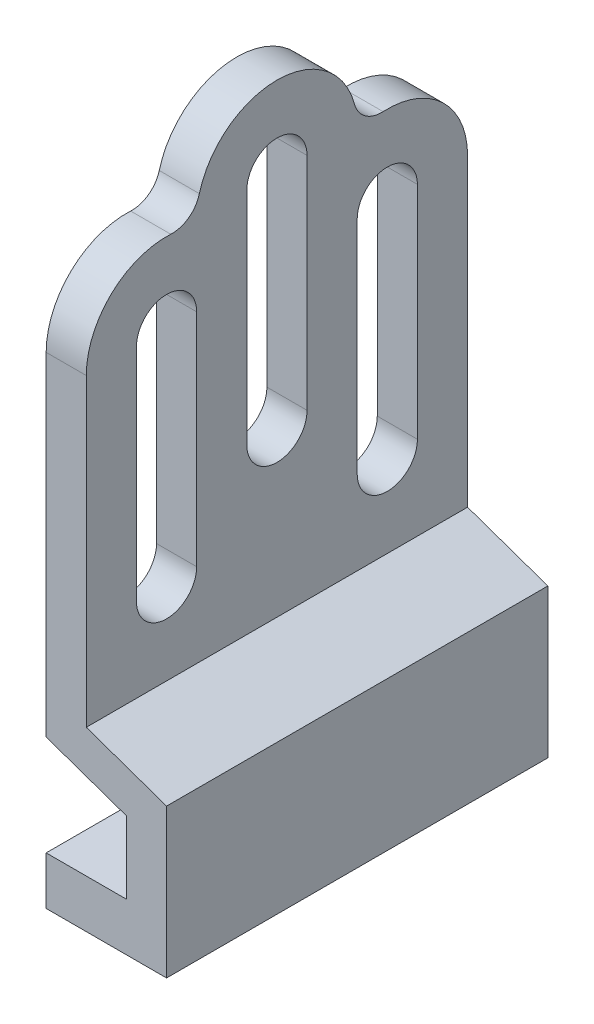
ISO-10303-21;
HEADER;
FILE_DESCRIPTION(('STEP AP214'),'2;1');
FILE_NAME('part.step','',(''),(''),'','','');
FILE_SCHEMA(('AUTOMOTIVE_DESIGN { 1 0 10303 214 1 1 1 1 }'));
ENDSEC;
DATA;
#1=APPLICATION_CONTEXT('core data for automotive mechanical design processes');
#2=APPLICATION_PROTOCOL_DEFINITION('international standard','automotive_design',2000,#1);
#3=PRODUCT_CONTEXT('',#1,'mechanical');
#4=PRODUCT('Part','Part','',(#3));
#5=PRODUCT_RELATED_PRODUCT_CATEGORY('part','',(#4));
#6=PRODUCT_DEFINITION_FORMATION('','',#4);
#7=PRODUCT_DEFINITION_CONTEXT('part definition',#1,'design');
#8=PRODUCT_DEFINITION('design','',#6,#7);
#9=PRODUCT_DEFINITION_SHAPE('','',#8);
#10=(LENGTH_UNIT() NAMED_UNIT(*) SI_UNIT(.MILLI.,.METRE.));
#11=(NAMED_UNIT(*) PLANE_ANGLE_UNIT() SI_UNIT($,.RADIAN.));
#12=(NAMED_UNIT(*) SI_UNIT($,.STERADIAN.) SOLID_ANGLE_UNIT());
#13=UNCERTAINTY_MEASURE_WITH_UNIT(LENGTH_MEASURE(1.E-05),#10,'distance_accuracy_value','');
#14=(GEOMETRIC_REPRESENTATION_CONTEXT(3) GLOBAL_UNCERTAINTY_ASSIGNED_CONTEXT((#13)) GLOBAL_UNIT_ASSIGNED_CONTEXT((#10,
#11,#12)) REPRESENTATION_CONTEXT('',''));
#15=CARTESIAN_POINT('',(0.,0.,0.));
#16=DIRECTION('',(0.,0.,1.));
#17=DIRECTION('',(1.,0.,0.));
#18=AXIS2_PLACEMENT_3D('',#15,#16,#17);
#19=CARTESIAN_POINT('',(-20.,44.0948100502085,47.5));
#20=DIRECTION('',(-1.,0.,0.));
#21=DIRECTION('',(0.,0.,1.));
#22=AXIS2_PLACEMENT_3D('',#19,#20,#21);
#23=PLANE('',#22);
#24=CARTESIAN_POINT('',(-20.,140.,0.));
#25=DIRECTION('',(1.,0.,0.));
#26=DIRECTION('',(0.,0.,-1.));
#27=AXIS2_PLACEMENT_3D('',#24,#25,#26);
#28=CIRCLE('',#27,20.);
#29=CARTESIAN_POINT('',(-20.,145.157767655643,-19.3234943219492));
#30=VERTEX_POINT('',#29);
#31=CARTESIAN_POINT('',(-20.,145.157767655643,19.3234943219492));
#32=VERTEX_POINT('',#31);
#33=EDGE_CURVE('E462',#30,#32,#28,.T.);
#34=ORIENTED_EDGE('',*,*,#33,.T.);
#35=CARTESIAN_POINT('',(-20.,146.962986335118,26.0867173346314));
#36=DIRECTION('',(1.,0.,0.));
#37=DIRECTION('',(0.,0.,-1.));
#38=AXIS2_PLACEMENT_3D('',#35,#36,#37);
#39=CIRCLE('',#38,7.);
#40=CARTESIAN_POINT('',(-20.,139.972582470458,26.4531239515788));
#41=VERTEX_POINT('',#40);
#42=EDGE_CURVE('E332',#32,#41,#39,.F.);
#43=ORIENTED_EDGE('',*,*,#42,.T.);
#44=CARTESIAN_POINT('',(-20.,120.,27.5));
#45=DIRECTION('',(1.,0.,0.));
#46=DIRECTION('',(0.,0.,-1.));
#47=AXIS2_PLACEMENT_3D('',#44,#45,#46);
#48=CIRCLE('',#47,20.);
#49=CARTESIAN_POINT('',(-20.,120.,47.5));
#50=VERTEX_POINT('',#49);
#51=EDGE_CURVE('E419',#41,#50,#48,.T.);
#52=ORIENTED_EDGE('',*,*,#51,.T.);
#53=DIRECTION('',(0.,1.,0.));
#54=VECTOR('',#53,1.);
#55=CARTESIAN_POINT('',(-20.,44.0948100502085,47.5));
#56=LINE('',#55,#54);
#57=CARTESIAN_POINT('',(-20.,44.0948100502085,47.5));
#58=VERTEX_POINT('',#57);
#59=EDGE_CURVE('E338',#58,#50,#56,.T.);
#60=ORIENTED_EDGE('',*,*,#59,.F.);
#61=DIRECTION('',(0.,0.,-1.));
#62=VECTOR('',#61,1.);
#63=CARTESIAN_POINT('',(-20.,44.0948100502085,47.5));
#64=LINE('',#63,#62);
#65=CARTESIAN_POINT('',(-20.,44.0948100502085,-47.5));
#66=VERTEX_POINT('',#65);
#67=EDGE_CURVE('E392',#58,#66,#64,.T.);
#68=ORIENTED_EDGE('',*,*,#67,.T.);
#69=DIRECTION('',(0.,1.,0.));
#70=VECTOR('',#69,1.);
#71=CARTESIAN_POINT('',(-20.,44.0948100502085,-47.5));
#72=LINE('',#71,#70);
#73=CARTESIAN_POINT('',(-20.,120.,-47.5));
#74=VERTEX_POINT('',#73);
#75=EDGE_CURVE('E367',#66,#74,#72,.T.);
#76=ORIENTED_EDGE('',*,*,#75,.T.);
#77=CARTESIAN_POINT('',(-20.,120.,-27.5));
#78=DIRECTION('',(1.,0.,0.));
#79=DIRECTION('',(0.,0.,-1.));
#80=AXIS2_PLACEMENT_3D('',#77,#78,#79);
#81=CIRCLE('',#80,20.);
#82=CARTESIAN_POINT('',(-20.,139.972582470458,-26.4531239515788));
#83=VERTEX_POINT('',#82);
#84=EDGE_CURVE('E468',#83,#74,#81,.F.);
#85=ORIENTED_EDGE('',*,*,#84,.F.);
#86=CARTESIAN_POINT('',(-20.,146.962986335118,-26.0867173346314));
#87=DIRECTION('',(1.,0.,0.));
#88=DIRECTION('',(0.,0.,-1.));
#89=AXIS2_PLACEMENT_3D('',#86,#87,#88);
#90=CIRCLE('',#89,7.);
#91=EDGE_CURVE('E464',#30,#83,#90,.T.);
#92=ORIENTED_EDGE('',*,*,#91,.F.);
#93=EDGE_LOOP('',(#34,#43,#52,#60,#68,#76,#85,#92));
#94=FACE_BOUND('',#93,.T.);
#95=CARTESIAN_POINT('',(-20.,65.,27.5));
#96=DIRECTION('',(1.,0.,0.));
#97=DIRECTION('',(0.,0.,-1.));
#98=AXIS2_PLACEMENT_3D('',#95,#96,#97);
#99=CIRCLE('',#98,7.50000000000001);
#100=CARTESIAN_POINT('',(-20.,65.,35.));
#101=VERTEX_POINT('',#100);
#102=CARTESIAN_POINT('',(-20.,65.,20.));
#103=VERTEX_POINT('',#102);
#104=EDGE_CURVE('E438',#101,#103,#99,.T.);
#105=ORIENTED_EDGE('',*,*,#104,.F.);
#106=DIRECTION('',(0.,-1.,0.));
#107=VECTOR('',#106,1.);
#108=CARTESIAN_POINT('',(-20.,0.,35.));
#109=LINE('',#108,#107);
#110=CARTESIAN_POINT('',(-20.,120.,35.));
#111=VERTEX_POINT('',#110);
#112=EDGE_CURVE('E168',#111,#101,#109,.T.);
#113=ORIENTED_EDGE('',*,*,#112,.F.);
#114=CARTESIAN_POINT('',(-20.,120.,27.5));
#115=DIRECTION('',(1.,0.,0.));
#116=DIRECTION('',(0.,0.,-1.));
#117=AXIS2_PLACEMENT_3D('',#114,#115,#116);
#118=CIRCLE('',#117,7.5);
#119=CARTESIAN_POINT('',(-20.,120.,20.));
#120=VERTEX_POINT('',#119);
#121=EDGE_CURVE('E443',#120,#111,#118,.T.);
#122=ORIENTED_EDGE('',*,*,#121,.F.);
#123=DIRECTION('',(0.,-1.,0.));
#124=VECTOR('',#123,1.);
#125=CARTESIAN_POINT('',(-20.,0.,20.));
#126=LINE('',#125,#124);
#127=EDGE_CURVE('E445',#120,#103,#126,.T.);
#128=ORIENTED_EDGE('',*,*,#127,.T.);
#129=EDGE_LOOP('',(#105,#113,#122,#128));
#130=FACE_BOUND('',#129,.T.);
#131=CARTESIAN_POINT('',(-20.,85.,0.));
#132=DIRECTION('',(1.,0.,0.));
#133=DIRECTION('',(0.,0.,-1.));
#134=AXIS2_PLACEMENT_3D('',#131,#132,#133);
#135=CIRCLE('',#134,7.5);
#136=CARTESIAN_POINT('',(-20.,85.,7.49999999999999));
#137=VERTEX_POINT('',#136);
#138=CARTESIAN_POINT('',(-20.,85.,-7.50000000000001));
#139=VERTEX_POINT('',#138);
#140=EDGE_CURVE('E489',#137,#139,#135,.T.);
#141=ORIENTED_EDGE('',*,*,#140,.F.);
#142=DIRECTION('',(0.,-1.,0.));
#143=VECTOR('',#142,1.);
#144=CARTESIAN_POINT('',(-20.,0.,7.49999999999998));
#145=LINE('',#144,#143);
#146=CARTESIAN_POINT('',(-20.,140.,7.5));
#147=VERTEX_POINT('',#146);
#148=EDGE_CURVE('E488',#147,#137,#145,.T.);
#149=ORIENTED_EDGE('',*,*,#148,.F.);
#150=CARTESIAN_POINT('',(-20.,140.,0.));
#151=DIRECTION('',(1.,0.,0.));
#152=DIRECTION('',(0.,0.,-1.));
#153=AXIS2_PLACEMENT_3D('',#150,#151,#152);
#154=CIRCLE('',#153,7.5);
#155=CARTESIAN_POINT('',(-20.,140.,-7.5));
#156=VERTEX_POINT('',#155);
#157=EDGE_CURVE('E497',#156,#147,#154,.T.);
#158=ORIENTED_EDGE('',*,*,#157,.F.);
#159=DIRECTION('',(0.,-1.,0.));
#160=VECTOR('',#159,1.);
#161=CARTESIAN_POINT('',(-20.,0.,-7.50000000000002));
#162=LINE('',#161,#160);
#163=EDGE_CURVE('E492',#156,#139,#162,.T.);
#164=ORIENTED_EDGE('',*,*,#163,.T.);
#165=EDGE_LOOP('',(#141,#149,#158,#164));
#166=FACE_BOUND('',#165,.T.);
#167=CARTESIAN_POINT('',(-20.,65.,-27.5));
#168=DIRECTION('',(1.,0.,0.));
#169=DIRECTION('',(0.,0.,-1.));
#170=AXIS2_PLACEMENT_3D('',#167,#168,#169);
#171=CIRCLE('',#170,7.50000000000001);
#172=CARTESIAN_POINT('',(-20.,65.,-35.));
#173=VERTEX_POINT('',#172);
#174=CARTESIAN_POINT('',(-20.,65.,-20.));
#175=VERTEX_POINT('',#174);
#176=EDGE_CURVE('E520',#173,#175,#171,.F.);
#177=ORIENTED_EDGE('',*,*,#176,.T.);
#178=DIRECTION('',(0.,-1.,0.));
#179=VECTOR('',#178,1.);
#180=CARTESIAN_POINT('',(-20.,0.,-20.));
#181=LINE('',#180,#179);
#182=CARTESIAN_POINT('',(-20.,120.,-20.));
#183=VERTEX_POINT('',#182);
#184=EDGE_CURVE('E528',#183,#175,#181,.T.);
#185=ORIENTED_EDGE('',*,*,#184,.F.);
#186=CARTESIAN_POINT('',(-20.,120.,-27.5));
#187=DIRECTION('',(1.,0.,0.));
#188=DIRECTION('',(0.,0.,-1.));
#189=AXIS2_PLACEMENT_3D('',#186,#187,#188);
#190=CIRCLE('',#189,7.5);
#191=CARTESIAN_POINT('',(-20.,120.,-35.));
#192=VERTEX_POINT('',#191);
#193=EDGE_CURVE('E522',#183,#192,#190,.F.);
#194=ORIENTED_EDGE('',*,*,#193,.T.);
#195=DIRECTION('',(0.,-1.,0.));
#196=VECTOR('',#195,1.);
#197=CARTESIAN_POINT('',(-20.,0.,-35.));
#198=LINE('',#197,#196);
#199=EDGE_CURVE('E518',#192,#173,#198,.T.);
#200=ORIENTED_EDGE('',*,*,#199,.T.);
#201=EDGE_LOOP('',(#177,#185,#194,#200));
#202=FACE_BOUND('',#201,.T.);
#203=ADVANCED_FACE('F150',(#94,#130,#166,#202),#23,.F.);
#204=CARTESIAN_POINT('',(-30.,160.,47.5));
#205=DIRECTION('',(1.,0.,0.));
#206=DIRECTION('',(0.,1.,0.));
#207=AXIS2_PLACEMENT_3D('',#204,#205,#206);
#208=PLANE('',#207);
#209=DIRECTION('',(0.,-1.,0.));
#210=VECTOR('',#209,1.);
#211=CARTESIAN_POINT('',(-30.,160.,47.5));
#212=LINE('',#211,#210);
#213=CARTESIAN_POINT('',(-30.,120.,47.5));
#214=VERTEX_POINT('',#213);
#215=CARTESIAN_POINT('',(-30.,37.,47.5));
#216=VERTEX_POINT('',#215);
#217=EDGE_CURVE('E340',#214,#216,#212,.T.);
#218=ORIENTED_EDGE('',*,*,#217,.F.);
#219=CARTESIAN_POINT('',(-30.,120.,27.5));
#220=DIRECTION('',(1.,0.,0.));
#221=DIRECTION('',(0.,1.,0.));
#222=AXIS2_PLACEMENT_3D('',#219,#220,#221);
#223=CIRCLE('',#222,20.);
#224=CARTESIAN_POINT('',(-30.,139.972582470458,26.4531239515788));
#225=VERTEX_POINT('',#224);
#226=EDGE_CURVE('E321',#214,#225,#223,.F.);
#227=ORIENTED_EDGE('',*,*,#226,.T.);
#228=CARTESIAN_POINT('',(-30.,146.962986335118,26.0867173346314));
#229=DIRECTION('',(1.,0.,0.));
#230=DIRECTION('',(0.,1.,0.));
#231=AXIS2_PLACEMENT_3D('',#228,#229,#230);
#232=CIRCLE('',#231,7.);
#233=CARTESIAN_POINT('',(-30.,145.157767655643,19.3234943219492));
#234=VERTEX_POINT('',#233);
#235=EDGE_CURVE('E335',#225,#234,#232,.T.);
#236=ORIENTED_EDGE('',*,*,#235,.T.);
#237=CARTESIAN_POINT('',(-30.,140.,0.));
#238=DIRECTION('',(1.,0.,0.));
#239=DIRECTION('',(0.,1.,0.));
#240=AXIS2_PLACEMENT_3D('',#237,#238,#239);
#241=CIRCLE('',#240,20.);
#242=CARTESIAN_POINT('',(-30.,145.157767655643,-19.3234943219492));
#243=VERTEX_POINT('',#242);
#244=EDGE_CURVE('E165',#234,#243,#241,.F.);
#245=ORIENTED_EDGE('',*,*,#244,.T.);
#246=CARTESIAN_POINT('',(-30.,146.962986335118,-26.0867173346314));
#247=DIRECTION('',(1.,0.,0.));
#248=DIRECTION('',(0.,1.,0.));
#249=AXIS2_PLACEMENT_3D('',#246,#247,#248);
#250=CIRCLE('',#249,7.);
#251=CARTESIAN_POINT('',(-30.,139.972582470458,-26.4531239515788));
#252=VERTEX_POINT('',#251);
#253=EDGE_CURVE('E473',#252,#243,#250,.F.);
#254=ORIENTED_EDGE('',*,*,#253,.F.);
#255=CARTESIAN_POINT('',(-30.,120.,-27.5));
#256=DIRECTION('',(1.,0.,0.));
#257=DIRECTION('',(0.,1.,0.));
#258=AXIS2_PLACEMENT_3D('',#255,#256,#257);
#259=CIRCLE('',#258,20.);
#260=CARTESIAN_POINT('',(-30.,120.,-47.5));
#261=VERTEX_POINT('',#260);
#262=EDGE_CURVE('E426',#261,#252,#259,.T.);
#263=ORIENTED_EDGE('',*,*,#262,.F.);
#264=DIRECTION('',(0.,-1.,0.));
#265=VECTOR('',#264,1.);
#266=CARTESIAN_POINT('',(-30.,160.,-47.5));
#267=LINE('',#266,#265);
#268=CARTESIAN_POINT('',(-30.,37.,-47.5));
#269=VERTEX_POINT('',#268);
#270=EDGE_CURVE('E373',#261,#269,#267,.T.);
#271=ORIENTED_EDGE('',*,*,#270,.T.);
#272=DIRECTION('',(0.,0.,-1.));
#273=VECTOR('',#272,1.);
#274=CARTESIAN_POINT('',(-30.,37.,47.5));
#275=LINE('',#274,#273);
#276=EDGE_CURVE('E347',#216,#269,#275,.T.);
#277=ORIENTED_EDGE('',*,*,#276,.F.);
#278=EDGE_LOOP('',(#218,#227,#236,#245,#254,#263,#271,#277));
#279=FACE_BOUND('',#278,.T.);
#280=CARTESIAN_POINT('',(-30.,120.,27.5));
#281=DIRECTION('',(1.,0.,0.));
#282=DIRECTION('',(0.,1.,0.));
#283=AXIS2_PLACEMENT_3D('',#280,#281,#282);
#284=CIRCLE('',#283,7.5);
#285=CARTESIAN_POINT('',(-30.,120.,35.));
#286=VERTEX_POINT('',#285);
#287=CARTESIAN_POINT('',(-30.,120.,20.));
#288=VERTEX_POINT('',#287);
#289=EDGE_CURVE('E431',#286,#288,#284,.F.);
#290=ORIENTED_EDGE('',*,*,#289,.F.);
#291=DIRECTION('',(0.,1.,0.));
#292=VECTOR('',#291,1.);
#293=CARTESIAN_POINT('',(-30.,0.,35.));
#294=LINE('',#293,#292);
#295=CARTESIAN_POINT('',(-30.,65.,35.));
#296=VERTEX_POINT('',#295);
#297=EDGE_CURVE('E434',#296,#286,#294,.T.);
#298=ORIENTED_EDGE('',*,*,#297,.F.);
#299=CARTESIAN_POINT('',(-30.,65.,27.5));
#300=DIRECTION('',(1.,0.,0.));
#301=DIRECTION('',(0.,1.,0.));
#302=AXIS2_PLACEMENT_3D('',#299,#300,#301);
#303=CIRCLE('',#302,7.50000000000001);
#304=CARTESIAN_POINT('',(-30.,65.,20.));
#305=VERTEX_POINT('',#304);
#306=EDGE_CURVE('E365',#305,#296,#303,.F.);
#307=ORIENTED_EDGE('',*,*,#306,.F.);
#308=DIRECTION('',(0.,1.,0.));
#309=VECTOR('',#308,1.);
#310=CARTESIAN_POINT('',(-30.,0.,20.));
#311=LINE('',#310,#309);
#312=EDGE_CURVE('E428',#305,#288,#311,.T.);
#313=ORIENTED_EDGE('',*,*,#312,.T.);
#314=EDGE_LOOP('',(#290,#298,#307,#313));
#315=FACE_BOUND('',#314,.T.);
#316=CARTESIAN_POINT('',(-30.,140.,0.));
#317=DIRECTION('',(1.,0.,0.));
#318=DIRECTION('',(0.,1.,0.));
#319=AXIS2_PLACEMENT_3D('',#316,#317,#318);
#320=CIRCLE('',#319,7.5);
#321=CARTESIAN_POINT('',(-30.,140.,7.5));
#322=VERTEX_POINT('',#321);
#323=CARTESIAN_POINT('',(-30.,140.,-7.5));
#324=VERTEX_POINT('',#323);
#325=EDGE_CURVE('E481',#322,#324,#320,.F.);
#326=ORIENTED_EDGE('',*,*,#325,.F.);
#327=DIRECTION('',(0.,1.,0.));
#328=VECTOR('',#327,1.);
#329=CARTESIAN_POINT('',(-30.,0.,7.49999999999998));
#330=LINE('',#329,#328);
#331=CARTESIAN_POINT('',(-30.,85.,7.49999999999999));
#332=VERTEX_POINT('',#331);
#333=EDGE_CURVE('E484',#332,#322,#330,.T.);
#334=ORIENTED_EDGE('',*,*,#333,.F.);
#335=CARTESIAN_POINT('',(-30.,85.,0.));
#336=DIRECTION('',(1.,0.,0.));
#337=DIRECTION('',(0.,1.,0.));
#338=AXIS2_PLACEMENT_3D('',#335,#336,#337);
#339=CIRCLE('',#338,7.5);
#340=CARTESIAN_POINT('',(-30.,85.,-7.50000000000001));
#341=VERTEX_POINT('',#340);
#342=EDGE_CURVE('E435',#341,#332,#339,.F.);
#343=ORIENTED_EDGE('',*,*,#342,.F.);
#344=DIRECTION('',(0.,1.,0.));
#345=VECTOR('',#344,1.);
#346=CARTESIAN_POINT('',(-30.,0.,-7.50000000000002));
#347=LINE('',#346,#345);
#348=EDGE_CURVE('E476',#341,#324,#347,.T.);
#349=ORIENTED_EDGE('',*,*,#348,.T.);
#350=EDGE_LOOP('',(#326,#334,#343,#349));
#351=FACE_BOUND('',#350,.T.);
#352=CARTESIAN_POINT('',(-30.,65.,-27.5));
#353=DIRECTION('',(1.,0.,0.));
#354=DIRECTION('',(0.,1.,0.));
#355=AXIS2_PLACEMENT_3D('',#352,#353,#354);
#356=CIRCLE('',#355,7.50000000000001);
#357=CARTESIAN_POINT('',(-30.,65.,-20.));
#358=VERTEX_POINT('',#357);
#359=CARTESIAN_POINT('',(-30.,65.,-35.));
#360=VERTEX_POINT('',#359);
#361=EDGE_CURVE('E514',#358,#360,#356,.T.);
#362=ORIENTED_EDGE('',*,*,#361,.T.);
#363=DIRECTION('',(0.,1.,0.));
#364=VECTOR('',#363,1.);
#365=CARTESIAN_POINT('',(-30.,0.,-35.));
#366=LINE('',#365,#364);
#367=CARTESIAN_POINT('',(-30.,120.,-35.));
#368=VERTEX_POINT('',#367);
#369=EDGE_CURVE('E485',#360,#368,#366,.T.);
#370=ORIENTED_EDGE('',*,*,#369,.T.);
#371=CARTESIAN_POINT('',(-30.,120.,-27.5));
#372=DIRECTION('',(1.,0.,0.));
#373=DIRECTION('',(0.,1.,0.));
#374=AXIS2_PLACEMENT_3D('',#371,#372,#373);
#375=CIRCLE('',#374,7.5);
#376=CARTESIAN_POINT('',(-30.,120.,-20.));
#377=VERTEX_POINT('',#376);
#378=EDGE_CURVE('E480',#368,#377,#375,.T.);
#379=ORIENTED_EDGE('',*,*,#378,.T.);
#380=DIRECTION('',(0.,1.,0.));
#381=VECTOR('',#380,1.);
#382=CARTESIAN_POINT('',(-30.,0.,-20.));
#383=LINE('',#382,#381);
#384=EDGE_CURVE('E515',#358,#377,#383,.T.);
#385=ORIENTED_EDGE('',*,*,#384,.F.);
#386=EDGE_LOOP('',(#362,#370,#379,#385));
#387=FACE_BOUND('',#386,.T.);
#388=ADVANCED_FACE('F342',(#279,#315,#351,#387),#208,.F.);
#389=CARTESIAN_POINT('',(-30.,0.,47.5));
#390=DIRECTION('',(1.,0.,0.));
#391=DIRECTION('',(0.,0.,-1.));
#392=AXIS2_PLACEMENT_3D('',#389,#390,#391);
#393=PLANE('',#392);
#394=DIRECTION('',(0.,-1.,0.));
#395=VECTOR('',#394,1.);
#396=CARTESIAN_POINT('',(-30.,0.,-47.5));
#397=LINE('',#396,#395);
#398=CARTESIAN_POINT('',(-30.,12.,-47.5));
#399=VERTEX_POINT('',#398);
#400=CARTESIAN_POINT('',(-30.,0.,-47.5));
#401=VERTEX_POINT('',#400);
#402=EDGE_CURVE('E356',#399,#401,#397,.T.);
#403=ORIENTED_EDGE('',*,*,#402,.T.);
#404=DIRECTION('',(0.,0.,-1.));
#405=VECTOR('',#404,1.);
#406=CARTESIAN_POINT('',(-30.,0.,47.5));
#407=LINE('',#406,#405);
#408=CARTESIAN_POINT('',(-30.,0.,47.5));
#409=VERTEX_POINT('',#408);
#410=EDGE_CURVE('E12',#409,#401,#407,.T.);
#411=ORIENTED_EDGE('',*,*,#410,.F.);
#412=DIRECTION('',(0.,-1.,0.));
#413=VECTOR('',#412,1.);
#414=CARTESIAN_POINT('',(-30.,0.,47.5));
#415=LINE('',#414,#413);
#416=CARTESIAN_POINT('',(-30.,12.,47.5));
#417=VERTEX_POINT('',#416);
#418=EDGE_CURVE('E381',#417,#409,#415,.T.);
#419=ORIENTED_EDGE('',*,*,#418,.F.);
#420=DIRECTION('',(0.,0.,-1.));
#421=VECTOR('',#420,1.);
#422=CARTESIAN_POINT('',(-30.,12.,47.5));
#423=LINE('',#422,#421);
#424=EDGE_CURVE('E360',#417,#399,#423,.T.);
#425=ORIENTED_EDGE('',*,*,#424,.T.);
#426=EDGE_LOOP('',(#403,#411,#419,#425));
#427=FACE_BOUND('',#426,.T.);
#428=ADVANCED_FACE('F149',(#427),#393,.F.);
#429=CARTESIAN_POINT('',(-30.,0.,47.5));
#430=DIRECTION('',(0.,1.,0.));
#431=DIRECTION('',(0.,0.,1.));
#432=AXIS2_PLACEMENT_3D('',#429,#430,#431);
#433=PLANE('',#432);
#434=DIRECTION('',(1.,0.,0.));
#435=VECTOR('',#434,1.);
#436=CARTESIAN_POINT('',(-30.,0.,-47.5));
#437=LINE('',#436,#435);
#438=CARTESIAN_POINT('',(0.,0.,-47.5));
#439=VERTEX_POINT('',#438);
#440=EDGE_CURVE('E361',#401,#439,#437,.T.);
#441=ORIENTED_EDGE('',*,*,#440,.T.);
#442=DIRECTION('',(0.,0.,-1.));
#443=VECTOR('',#442,1.);
#444=CARTESIAN_POINT('',(0.,0.,47.5));
#445=LINE('',#444,#443);
#446=CARTESIAN_POINT('',(0.,0.,47.5));
#447=VERTEX_POINT('',#446);
#448=EDGE_CURVE('E154',#447,#439,#445,.T.);
#449=ORIENTED_EDGE('',*,*,#448,.F.);
#450=DIRECTION('',(1.,0.,0.));
#451=VECTOR('',#450,1.);
#452=CARTESIAN_POINT('',(-30.,0.,47.5));
#453=LINE('',#452,#451);
#454=EDGE_CURVE('E545',#409,#447,#453,.T.);
#455=ORIENTED_EDGE('',*,*,#454,.F.);
#456=ORIENTED_EDGE('',*,*,#410,.T.);
#457=EDGE_LOOP('',(#441,#449,#455,#456));
#458=FACE_BOUND('',#457,.T.);
#459=ADVANCED_FACE('F546',(#458),#433,.F.);
#460=CARTESIAN_POINT('',(0.,0.,47.5));
#461=DIRECTION('',(-1.,0.,0.));
#462=DIRECTION('',(0.,-1.,0.));
#463=AXIS2_PLACEMENT_3D('',#460,#461,#462);
#464=PLANE('',#463);
#465=DIRECTION('',(0.,1.,0.));
#466=VECTOR('',#465,1.);
#467=CARTESIAN_POINT('',(0.,0.,-47.5));
#468=LINE('',#467,#466);
#469=CARTESIAN_POINT('',(0.,37.0948100502085,-47.5));
#470=VERTEX_POINT('',#469);
#471=EDGE_CURVE('E368',#439,#470,#468,.T.);
#472=ORIENTED_EDGE('',*,*,#471,.T.);
#473=DIRECTION('',(0.,0.,-1.));
#474=VECTOR('',#473,1.);
#475=CARTESIAN_POINT('',(0.,37.0948100502085,47.5));
#476=LINE('',#475,#474);
#477=CARTESIAN_POINT('',(0.,37.0948100502085,47.5));
#478=VERTEX_POINT('',#477);
#479=EDGE_CURVE('E391',#478,#470,#476,.T.);
#480=ORIENTED_EDGE('',*,*,#479,.F.);
#481=DIRECTION('',(0.,1.,0.));
#482=VECTOR('',#481,1.);
#483=CARTESIAN_POINT('',(0.,0.,47.5));
#484=LINE('',#483,#482);
#485=EDGE_CURVE('E401',#447,#478,#484,.T.);
#486=ORIENTED_EDGE('',*,*,#485,.F.);
#487=ORIENTED_EDGE('',*,*,#448,.T.);
#488=EDGE_LOOP('',(#472,#480,#486,#487));
#489=FACE_BOUND('',#488,.T.);
#490=ADVANCED_FACE('F402',(#489),#464,.F.);
#491=CARTESIAN_POINT('',(0.,37.0948100502085,47.5));
#492=DIRECTION('',(-0.330350424728106,-0.943858356366018,0.));
#493=DIRECTION('',(0.943858356366018,-0.330350424728106,0.));
#494=AXIS2_PLACEMENT_3D('',#491,#492,#493);
#495=PLANE('',#494);
#496=DIRECTION('',(-0.943858356366017,0.330350424728106,0.));
#497=VECTOR('',#496,1.);
#498=CARTESIAN_POINT('',(0.,37.0948100502085,-47.5));
#499=LINE('',#498,#497);
#500=EDGE_CURVE('E366',#470,#66,#499,.T.);
#501=ORIENTED_EDGE('',*,*,#500,.T.);
#502=ORIENTED_EDGE('',*,*,#67,.F.);
#503=DIRECTION('',(-0.943858356366017,0.330350424728106,0.));
#504=VECTOR('',#503,1.);
#505=CARTESIAN_POINT('',(0.,37.0948100502085,47.5));
#506=LINE('',#505,#504);
#507=EDGE_CURVE('E355',#478,#58,#506,.T.);
#508=ORIENTED_EDGE('',*,*,#507,.F.);
#509=ORIENTED_EDGE('',*,*,#479,.T.);
#510=EDGE_LOOP('',(#501,#502,#508,#509));
#511=FACE_BOUND('',#510,.T.);
#512=ADVANCED_FACE('F415',(#511),#495,.F.);
#513=CARTESIAN_POINT('',(-30.,37.,47.5));
#514=DIRECTION('',(0.330350424728106,0.943858356366017,0.));
#515=DIRECTION('',(-0.943858356366018,0.330350424728106,0.));
#516=AXIS2_PLACEMENT_3D('',#513,#514,#515);
#517=PLANE('',#516);
#518=DIRECTION('',(0.943858356366017,-0.330350424728106,0.));
#519=VECTOR('',#518,1.);
#520=CARTESIAN_POINT('',(-30.,37.,-47.5));
#521=LINE('',#520,#519);
#522=CARTESIAN_POINT('',(-9.99999999999999,30.,-47.5));
#523=VERTEX_POINT('',#522);
#524=EDGE_CURVE('E374',#269,#523,#521,.T.);
#525=ORIENTED_EDGE('',*,*,#524,.T.);
#526=DIRECTION('',(0.,0.,-1.));
#527=VECTOR('',#526,1.);
#528=CARTESIAN_POINT('',(-9.99999999999999,30.,47.5));
#529=LINE('',#528,#527);
#530=CARTESIAN_POINT('',(-9.99999999999999,30.,47.5));
#531=VERTEX_POINT('',#530);
#532=EDGE_CURVE('E390',#531,#523,#529,.T.);
#533=ORIENTED_EDGE('',*,*,#532,.F.);
#534=DIRECTION('',(0.943858356366017,-0.330350424728106,0.));
#535=VECTOR('',#534,1.);
#536=CARTESIAN_POINT('',(-30.,37.,47.5));
#537=LINE('',#536,#535);
#538=EDGE_CURVE('E346',#216,#531,#537,.T.);
#539=ORIENTED_EDGE('',*,*,#538,.F.);
#540=ORIENTED_EDGE('',*,*,#276,.T.);
#541=EDGE_LOOP('',(#525,#533,#539,#540));
#542=FACE_BOUND('',#541,.T.);
#543=ADVANCED_FACE('F563',(#542),#517,.F.);
#544=CARTESIAN_POINT('',(-9.99999999999999,30.,47.5));
#545=DIRECTION('',(1.,0.,0.));
#546=DIRECTION('',(0.,0.,-1.));
#547=AXIS2_PLACEMENT_3D('',#544,#545,#546);
#548=PLANE('',#547);
#549=DIRECTION('',(0.,-1.,0.));
#550=VECTOR('',#549,1.);
#551=CARTESIAN_POINT('',(-9.99999999999999,30.,-47.5));
#552=LINE('',#551,#550);
#553=CARTESIAN_POINT('',(-9.99999999999999,12.,-47.5));
#554=VERTEX_POINT('',#553);
#555=EDGE_CURVE('E380',#523,#554,#552,.T.);
#556=ORIENTED_EDGE('',*,*,#555,.T.);
#557=DIRECTION('',(0.,0.,-1.));
#558=VECTOR('',#557,1.);
#559=CARTESIAN_POINT('',(-9.99999999999999,12.,47.5));
#560=LINE('',#559,#558);
#561=CARTESIAN_POINT('',(-9.99999999999999,12.,47.5));
#562=VERTEX_POINT('',#561);
#563=EDGE_CURVE('E383',#562,#554,#560,.T.);
#564=ORIENTED_EDGE('',*,*,#563,.F.);
#565=DIRECTION('',(0.,-1.,0.));
#566=VECTOR('',#565,1.);
#567=CARTESIAN_POINT('',(-9.99999999999999,30.,47.5));
#568=LINE('',#567,#566);
#569=EDGE_CURVE('E348',#531,#562,#568,.T.);
#570=ORIENTED_EDGE('',*,*,#569,.F.);
#571=ORIENTED_EDGE('',*,*,#532,.T.);
#572=EDGE_LOOP('',(#556,#564,#570,#571));
#573=FACE_BOUND('',#572,.T.);
#574=ADVANCED_FACE('F559',(#573),#548,.F.);
#575=CARTESIAN_POINT('',(-9.99999999999999,12.,47.5));
#576=DIRECTION('',(0.,-1.,0.));
#577=DIRECTION('',(1.,0.,0.));
#578=AXIS2_PLACEMENT_3D('',#575,#576,#577);
#579=PLANE('',#578);
#580=DIRECTION('',(-1.,0.,0.));
#581=VECTOR('',#580,1.);
#582=CARTESIAN_POINT('',(-9.99999999999999,12.,-47.5));
#583=LINE('',#582,#581);
#584=EDGE_CURVE('E377',#554,#399,#583,.T.);
#585=ORIENTED_EDGE('',*,*,#584,.T.);
#586=ORIENTED_EDGE('',*,*,#424,.F.);
#587=DIRECTION('',(-1.,0.,0.));
#588=VECTOR('',#587,1.);
#589=CARTESIAN_POINT('',(-9.99999999999999,12.,47.5));
#590=LINE('',#589,#588);
#591=EDGE_CURVE('E359',#562,#417,#590,.T.);
#592=ORIENTED_EDGE('',*,*,#591,.F.);
#593=ORIENTED_EDGE('',*,*,#563,.T.);
#594=EDGE_LOOP('',(#585,#586,#592,#593));
#595=FACE_BOUND('',#594,.T.);
#596=ADVANCED_FACE('F554',(#595),#579,.F.);
#597=CARTESIAN_POINT('',(0.,0.,47.5));
#598=DIRECTION('',(0.,0.,1.));
#599=DIRECTION('',(1.,0.,0.));
#600=AXIS2_PLACEMENT_3D('',#597,#598,#599);
#601=PLANE('',#600);
#602=DIRECTION('',(1.,0.,0.));
#603=VECTOR('',#602,1.);
#604=CARTESIAN_POINT('',(-30.001,120.,47.5));
#605=LINE('',#604,#603);
#606=EDGE_CURVE('E324',#214,#50,#605,.T.);
#607=ORIENTED_EDGE('',*,*,#606,.F.);
#608=ORIENTED_EDGE('',*,*,#217,.T.);
#609=ORIENTED_EDGE('',*,*,#538,.T.);
#610=ORIENTED_EDGE('',*,*,#569,.T.);
#611=ORIENTED_EDGE('',*,*,#591,.T.);
#612=ORIENTED_EDGE('',*,*,#418,.T.);
#613=ORIENTED_EDGE('',*,*,#454,.T.);
#614=ORIENTED_EDGE('',*,*,#485,.T.);
#615=ORIENTED_EDGE('',*,*,#507,.T.);
#616=ORIENTED_EDGE('',*,*,#59,.T.);
#617=EDGE_LOOP('',(#607,#608,#609,#610,#611,#612,#613,#614,#615,#616));
#618=FACE_BOUND('',#617,.T.);
#619=ADVANCED_FACE('F337',(#618),#601,.T.);
#620=CARTESIAN_POINT('',(0.,0.,-47.5));
#621=DIRECTION('',(0.,0.,1.));
#622=DIRECTION('',(1.,0.,0.));
#623=AXIS2_PLACEMENT_3D('',#620,#621,#622);
#624=PLANE('',#623);
#625=ORIENTED_EDGE('',*,*,#270,.F.);
#626=DIRECTION('',(1.,0.,0.));
#627=VECTOR('',#626,1.);
#628=CARTESIAN_POINT('',(-30.001,120.,-47.5));
#629=LINE('',#628,#627);
#630=EDGE_CURVE('E470',#261,#74,#629,.T.);
#631=ORIENTED_EDGE('',*,*,#630,.T.);
#632=ORIENTED_EDGE('',*,*,#75,.F.);
#633=ORIENTED_EDGE('',*,*,#500,.F.);
#634=ORIENTED_EDGE('',*,*,#471,.F.);
#635=ORIENTED_EDGE('',*,*,#440,.F.);
#636=ORIENTED_EDGE('',*,*,#402,.F.);
#637=ORIENTED_EDGE('',*,*,#584,.F.);
#638=ORIENTED_EDGE('',*,*,#555,.F.);
#639=ORIENTED_EDGE('',*,*,#524,.F.);
#640=EDGE_LOOP('',(#625,#631,#632,#633,#634,#635,#636,#637,#638,#639));
#641=FACE_BOUND('',#640,.T.);
#642=ADVANCED_FACE('F409',(#641),#624,.F.);
#643=CARTESIAN_POINT('',(-30.001,0.,7.49999999999998));
#644=DIRECTION('',(0.,0.,1.));
#645=DIRECTION('',(0.,-1.,0.));
#646=AXIS2_PLACEMENT_3D('',#643,#644,#645);
#647=PLANE('',#646);
#648=ORIENTED_EDGE('',*,*,#333,.T.);
#649=DIRECTION('',(1.,0.,0.));
#650=VECTOR('',#649,1.);
#651=CARTESIAN_POINT('',(-30.001,140.,7.5));
#652=LINE('',#651,#650);
#653=EDGE_CURVE('E498',#322,#147,#652,.T.);
#654=ORIENTED_EDGE('',*,*,#653,.T.);
#655=ORIENTED_EDGE('',*,*,#148,.T.);
#656=DIRECTION('',(1.,0.,0.));
#657=VECTOR('',#656,1.);
#658=CARTESIAN_POINT('',(-30.001,85.,7.49999999999999));
#659=LINE('',#658,#657);
#660=EDGE_CURVE('E496',#332,#137,#659,.T.);
#661=ORIENTED_EDGE('',*,*,#660,.F.);
#662=EDGE_LOOP('',(#648,#654,#655,#661));
#663=FACE_BOUND('',#662,.T.);
#664=ADVANCED_FACE('F660',(#663),#647,.F.);
#665=CARTESIAN_POINT('',(-30.001,140.,0.));
#666=DIRECTION('',(1.,0.,0.));
#667=DIRECTION('',(0.,0.,-1.));
#668=AXIS2_PLACEMENT_3D('',#665,#666,#667);
#669=CYLINDRICAL_SURFACE('',#668,7.5);
#670=ORIENTED_EDGE('',*,*,#325,.T.);
#671=DIRECTION('',(1.,0.,0.));
#672=VECTOR('',#671,1.);
#673=CARTESIAN_POINT('',(-30.001,140.,-7.5));
#674=LINE('',#673,#672);
#675=EDGE_CURVE('E505',#324,#156,#674,.T.);
#676=ORIENTED_EDGE('',*,*,#675,.T.);
#677=ORIENTED_EDGE('',*,*,#157,.T.);
#678=ORIENTED_EDGE('',*,*,#653,.F.);
#679=EDGE_LOOP('',(#670,#676,#677,#678));
#680=FACE_BOUND('',#679,.T.);
#681=ADVANCED_FACE('F671',(#680),#669,.F.);
#682=CARTESIAN_POINT('',(-30.001,0.,-7.50000000000002));
#683=DIRECTION('',(0.,0.,1.));
#684=DIRECTION('',(0.,-1.,0.));
#685=AXIS2_PLACEMENT_3D('',#682,#683,#684);
#686=PLANE('',#685);
#687=DIRECTION('',(1.,0.,0.));
#688=VECTOR('',#687,1.);
#689=CARTESIAN_POINT('',(-30.001,85.,-7.50000000000001));
#690=LINE('',#689,#688);
#691=EDGE_CURVE('E501',#341,#139,#690,.T.);
#692=ORIENTED_EDGE('',*,*,#691,.T.);
#693=ORIENTED_EDGE('',*,*,#163,.F.);
#694=ORIENTED_EDGE('',*,*,#675,.F.);
#695=ORIENTED_EDGE('',*,*,#348,.F.);
#696=EDGE_LOOP('',(#692,#693,#694,#695));
#697=FACE_BOUND('',#696,.T.);
#698=ADVANCED_FACE('F683',(#697),#686,.T.);
#699=CARTESIAN_POINT('',(-30.001,85.,0.));
#700=DIRECTION('',(1.,0.,0.));
#701=DIRECTION('',(0.,0.,-1.));
#702=AXIS2_PLACEMENT_3D('',#699,#700,#701);
#703=CYLINDRICAL_SURFACE('',#702,7.5);
#704=ORIENTED_EDGE('',*,*,#342,.T.);
#705=ORIENTED_EDGE('',*,*,#660,.T.);
#706=ORIENTED_EDGE('',*,*,#140,.T.);
#707=ORIENTED_EDGE('',*,*,#691,.F.);
#708=EDGE_LOOP('',(#704,#705,#706,#707));
#709=FACE_BOUND('',#708,.T.);
#710=ADVANCED_FACE('F694',(#709),#703,.F.);
#711=CARTESIAN_POINT('',(-30.001,65.,-27.5));
#712=DIRECTION('',(1.,0.,0.));
#713=DIRECTION('',(0.,0.,-1.));
#714=AXIS2_PLACEMENT_3D('',#711,#712,#713);
#715=CYLINDRICAL_SURFACE('',#714,7.50000000000001);
#716=DIRECTION('',(1.,0.,0.));
#717=VECTOR('',#716,1.);
#718=CARTESIAN_POINT('',(-30.001,65.,-20.));
#719=LINE('',#718,#717);
#720=EDGE_CURVE('E529',#358,#175,#719,.T.);
#721=ORIENTED_EDGE('',*,*,#720,.T.);
#722=ORIENTED_EDGE('',*,*,#176,.F.);
#723=DIRECTION('',(1.,0.,0.));
#724=VECTOR('',#723,1.);
#725=CARTESIAN_POINT('',(-30.001,65.,-35.));
#726=LINE('',#725,#724);
#727=EDGE_CURVE('E530',#360,#173,#726,.T.);
#728=ORIENTED_EDGE('',*,*,#727,.F.);
#729=ORIENTED_EDGE('',*,*,#361,.F.);
#730=EDGE_LOOP('',(#721,#722,#728,#729));
#731=FACE_BOUND('',#730,.T.);
#732=ADVANCED_FACE('F704',(#731),#715,.F.);
#733=CARTESIAN_POINT('',(-30.001,0.,-20.));
#734=DIRECTION('',(0.,0.,1.));
#735=DIRECTION('',(0.,-1.,0.));
#736=AXIS2_PLACEMENT_3D('',#733,#734,#735);
#737=PLANE('',#736);
#738=ORIENTED_EDGE('',*,*,#384,.T.);
#739=DIRECTION('',(1.,0.,0.));
#740=VECTOR('',#739,1.);
#741=CARTESIAN_POINT('',(-30.001,120.,-20.));
#742=LINE('',#741,#740);
#743=EDGE_CURVE('E535',#377,#183,#742,.T.);
#744=ORIENTED_EDGE('',*,*,#743,.T.);
#745=ORIENTED_EDGE('',*,*,#184,.T.);
#746=ORIENTED_EDGE('',*,*,#720,.F.);
#747=EDGE_LOOP('',(#738,#744,#745,#746));
#748=FACE_BOUND('',#747,.T.);
#749=ADVANCED_FACE('F714',(#748),#737,.F.);
#750=CARTESIAN_POINT('',(-30.001,120.,-27.5));
#751=DIRECTION('',(1.,0.,0.));
#752=DIRECTION('',(0.,0.,-1.));
#753=AXIS2_PLACEMENT_3D('',#750,#751,#752);
#754=CYLINDRICAL_SURFACE('',#753,7.5);
#755=DIRECTION('',(1.,0.,0.));
#756=VECTOR('',#755,1.);
#757=CARTESIAN_POINT('',(-30.001,120.,-35.));
#758=LINE('',#757,#756);
#759=EDGE_CURVE('E534',#368,#192,#758,.T.);
#760=ORIENTED_EDGE('',*,*,#759,.T.);
#761=ORIENTED_EDGE('',*,*,#193,.F.);
#762=ORIENTED_EDGE('',*,*,#743,.F.);
#763=ORIENTED_EDGE('',*,*,#378,.F.);
#764=EDGE_LOOP('',(#760,#761,#762,#763));
#765=FACE_BOUND('',#764,.T.);
#766=ADVANCED_FACE('F723',(#765),#754,.F.);
#767=CARTESIAN_POINT('',(-30.001,0.,-35.));
#768=DIRECTION('',(0.,0.,1.));
#769=DIRECTION('',(1.,0.,0.));
#770=AXIS2_PLACEMENT_3D('',#767,#768,#769);
#771=PLANE('',#770);
#772=ORIENTED_EDGE('',*,*,#727,.T.);
#773=ORIENTED_EDGE('',*,*,#199,.F.);
#774=ORIENTED_EDGE('',*,*,#759,.F.);
#775=ORIENTED_EDGE('',*,*,#369,.F.);
#776=EDGE_LOOP('',(#772,#773,#774,#775));
#777=FACE_BOUND('',#776,.T.);
#778=ADVANCED_FACE('F733',(#777),#771,.T.);
#779=CARTESIAN_POINT('',(-30.001,0.,35.));
#780=DIRECTION('',(0.,0.,1.));
#781=DIRECTION('',(1.,0.,0.));
#782=AXIS2_PLACEMENT_3D('',#779,#780,#781);
#783=PLANE('',#782);
#784=ORIENTED_EDGE('',*,*,#297,.T.);
#785=DIRECTION('',(1.,0.,0.));
#786=VECTOR('',#785,1.);
#787=CARTESIAN_POINT('',(-30.001,120.,35.));
#788=LINE('',#787,#786);
#789=EDGE_CURVE('E446',#286,#111,#788,.T.);
#790=ORIENTED_EDGE('',*,*,#789,.T.);
#791=ORIENTED_EDGE('',*,*,#112,.T.);
#792=DIRECTION('',(1.,0.,0.));
#793=VECTOR('',#792,1.);
#794=CARTESIAN_POINT('',(-30.001,65.,35.));
#795=LINE('',#794,#793);
#796=EDGE_CURVE('E449',#296,#101,#795,.T.);
#797=ORIENTED_EDGE('',*,*,#796,.F.);
#798=EDGE_LOOP('',(#784,#790,#791,#797));
#799=FACE_BOUND('',#798,.T.);
#800=ADVANCED_FACE('F741',(#799),#783,.F.);
#801=CARTESIAN_POINT('',(-30.001,120.,27.5));
#802=DIRECTION('',(1.,0.,0.));
#803=DIRECTION('',(0.,0.,-1.));
#804=AXIS2_PLACEMENT_3D('',#801,#802,#803);
#805=CYLINDRICAL_SURFACE('',#804,7.5);
#806=ORIENTED_EDGE('',*,*,#289,.T.);
#807=DIRECTION('',(1.,0.,0.));
#808=VECTOR('',#807,1.);
#809=CARTESIAN_POINT('',(-30.001,120.,20.));
#810=LINE('',#809,#808);
#811=EDGE_CURVE('E453',#288,#120,#810,.T.);
#812=ORIENTED_EDGE('',*,*,#811,.T.);
#813=ORIENTED_EDGE('',*,*,#121,.T.);
#814=ORIENTED_EDGE('',*,*,#789,.F.);
#815=EDGE_LOOP('',(#806,#812,#813,#814));
#816=FACE_BOUND('',#815,.T.);
#817=ADVANCED_FACE('F752',(#816),#805,.F.);
#818=CARTESIAN_POINT('',(-30.001,0.,20.));
#819=DIRECTION('',(0.,0.,1.));
#820=DIRECTION('',(0.,-1.,0.));
#821=AXIS2_PLACEMENT_3D('',#818,#819,#820);
#822=PLANE('',#821);
#823=DIRECTION('',(1.,0.,0.));
#824=VECTOR('',#823,1.);
#825=CARTESIAN_POINT('',(-30.001,65.,20.));
#826=LINE('',#825,#824);
#827=EDGE_CURVE('E452',#305,#103,#826,.T.);
#828=ORIENTED_EDGE('',*,*,#827,.T.);
#829=ORIENTED_EDGE('',*,*,#127,.F.);
#830=ORIENTED_EDGE('',*,*,#811,.F.);
#831=ORIENTED_EDGE('',*,*,#312,.F.);
#832=EDGE_LOOP('',(#828,#829,#830,#831));
#833=FACE_BOUND('',#832,.T.);
#834=ADVANCED_FACE('F762',(#833),#822,.T.);
#835=CARTESIAN_POINT('',(-30.001,65.,27.5));
#836=DIRECTION('',(1.,0.,0.));
#837=DIRECTION('',(0.,0.,-1.));
#838=AXIS2_PLACEMENT_3D('',#835,#836,#837);
#839=CYLINDRICAL_SURFACE('',#838,7.50000000000001);
#840=ORIENTED_EDGE('',*,*,#306,.T.);
#841=ORIENTED_EDGE('',*,*,#796,.T.);
#842=ORIENTED_EDGE('',*,*,#104,.T.);
#843=ORIENTED_EDGE('',*,*,#827,.F.);
#844=EDGE_LOOP('',(#840,#841,#842,#843));
#845=FACE_BOUND('',#844,.T.);
#846=ADVANCED_FACE('F774',(#845),#839,.F.);
#847=CARTESIAN_POINT('',(-30.001,140.,0.));
#848=DIRECTION('',(1.,0.,0.));
#849=DIRECTION('',(0.,0.,-1.));
#850=AXIS2_PLACEMENT_3D('',#847,#848,#849);
#851=CYLINDRICAL_SURFACE('',#850,20.);
#852=ORIENTED_EDGE('',*,*,#244,.F.);
#853=DIRECTION('',(1.,0.,0.));
#854=VECTOR('',#853,1.);
#855=CARTESIAN_POINT('',(-30.001,145.157767655643,19.3234943219492));
#856=LINE('',#855,#854);
#857=EDGE_CURVE('E343',#234,#32,#856,.T.);
#858=ORIENTED_EDGE('',*,*,#857,.T.);
#859=ORIENTED_EDGE('',*,*,#33,.F.);
#860=DIRECTION('',(1.,0.,0.));
#861=VECTOR('',#860,1.);
#862=CARTESIAN_POINT('',(-30.001,145.157767655643,-19.3234943219492));
#863=LINE('',#862,#861);
#864=EDGE_CURVE('E467',#243,#30,#863,.T.);
#865=ORIENTED_EDGE('',*,*,#864,.F.);
#866=EDGE_LOOP('',(#852,#858,#859,#865));
#867=FACE_BOUND('',#866,.T.);
#868=ADVANCED_FACE('F568',(#867),#851,.T.);
#869=CARTESIAN_POINT('',(-30.001,120.,-27.5));
#870=DIRECTION('',(1.,0.,0.));
#871=DIRECTION('',(0.,0.,-1.));
#872=AXIS2_PLACEMENT_3D('',#869,#870,#871);
#873=CYLINDRICAL_SURFACE('',#872,20.);
#874=ORIENTED_EDGE('',*,*,#262,.T.);
#875=DIRECTION('',(1.,0.,0.));
#876=VECTOR('',#875,1.);
#877=CARTESIAN_POINT('',(-30.001,139.972582470458,-26.4531239515788));
#878=LINE('',#877,#876);
#879=EDGE_CURVE('E472',#252,#83,#878,.T.);
#880=ORIENTED_EDGE('',*,*,#879,.T.);
#881=ORIENTED_EDGE('',*,*,#84,.T.);
#882=ORIENTED_EDGE('',*,*,#630,.F.);
#883=EDGE_LOOP('',(#874,#880,#881,#882));
#884=FACE_BOUND('',#883,.T.);
#885=ADVANCED_FACE('F561',(#884),#873,.T.);
#886=CARTESIAN_POINT('',(-30.001,146.962986335118,-26.0867173346314));
#887=DIRECTION('',(1.,0.,0.));
#888=DIRECTION('',(0.,0.,-1.));
#889=AXIS2_PLACEMENT_3D('',#886,#887,#888);
#890=CYLINDRICAL_SURFACE('',#889,7.);
#891=ORIENTED_EDGE('',*,*,#253,.T.);
#892=ORIENTED_EDGE('',*,*,#864,.T.);
#893=ORIENTED_EDGE('',*,*,#91,.T.);
#894=ORIENTED_EDGE('',*,*,#879,.F.);
#895=EDGE_LOOP('',(#891,#892,#893,#894));
#896=FACE_BOUND('',#895,.T.);
#897=ADVANCED_FACE('F569',(#896),#890,.F.);
#898=CARTESIAN_POINT('',(-30.001,146.962986335118,26.0867173346314));
#899=DIRECTION('',(1.,0.,0.));
#900=DIRECTION('',(0.,0.,-1.));
#901=AXIS2_PLACEMENT_3D('',#898,#899,#900);
#902=CYLINDRICAL_SURFACE('',#901,7.);
#903=DIRECTION('',(1.,0.,0.));
#904=VECTOR('',#903,1.);
#905=CARTESIAN_POINT('',(-30.001,139.972582470458,26.4531239515788));
#906=LINE('',#905,#904);
#907=EDGE_CURVE('E330',#225,#41,#906,.T.);
#908=ORIENTED_EDGE('',*,*,#907,.T.);
#909=ORIENTED_EDGE('',*,*,#42,.F.);
#910=ORIENTED_EDGE('',*,*,#857,.F.);
#911=ORIENTED_EDGE('',*,*,#235,.F.);
#912=EDGE_LOOP('',(#908,#909,#910,#911));
#913=FACE_BOUND('',#912,.T.);
#914=ADVANCED_FACE('F575',(#913),#902,.F.);
#915=CARTESIAN_POINT('',(-30.001,120.,27.5));
#916=DIRECTION('',(1.,0.,0.));
#917=DIRECTION('',(0.,0.,-1.));
#918=AXIS2_PLACEMENT_3D('',#915,#916,#917);
#919=CYLINDRICAL_SURFACE('',#918,20.);
#920=ORIENTED_EDGE('',*,*,#606,.T.);
#921=ORIENTED_EDGE('',*,*,#51,.F.);
#922=ORIENTED_EDGE('',*,*,#907,.F.);
#923=ORIENTED_EDGE('',*,*,#226,.F.);
#924=EDGE_LOOP('',(#920,#921,#922,#923));
#925=FACE_BOUND('',#924,.T.);
#926=ADVANCED_FACE('F323',(#925),#919,.T.);
#927=CLOSED_SHELL('',(#203,#388,#428,#459,#490,#512,#543,#574,#596,#619,#642,#664,#681,#698,
#710,#732,#749,#766,#778,#800,#817,#834,#846,#868,#885,#897,#914,#926));
#928=MANIFOLD_SOLID_BREP('B2',#927);
#929=ADVANCED_BREP_SHAPE_REPRESENTATION('',(#18,#928),#14);
#930=SHAPE_DEFINITION_REPRESENTATION(#9,#929);
ENDSEC;
END-ISO-10303-21;
